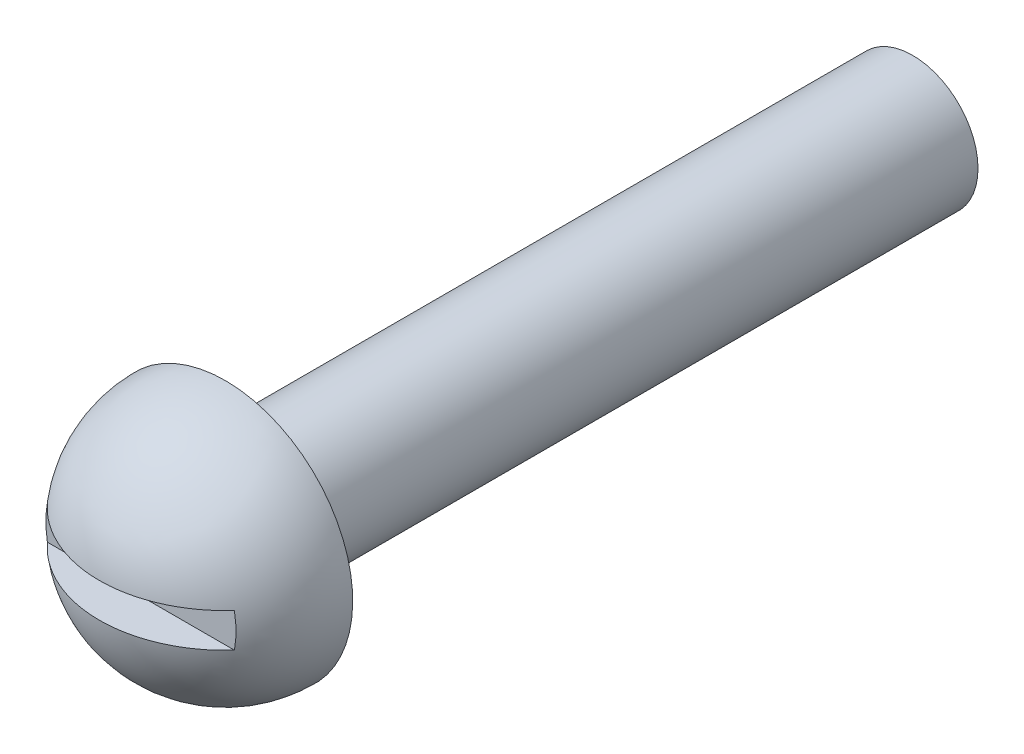
SolidWorks part; units mm, degrees
material "Plain Carbon Steel"
ref_plane "Front Plane" through (0, 0, 0) normal (0, 0, 1) x (1, 0, 0)
ref_plane "Top Plane" through (0, 0, 0) normal (0, 1, 0) x (1, 0, 0)
ref_plane "Right Plane" through (0, 0, 0) normal (1, 0, 0) x (0, 0, -1)
sketch "Shank Profile Ø0.19" plane through (0, 0, 0) normal (0, 0, 1) x (1, 0, 0)
  circle A0 centre (0, 0) radius 2.413
  dimension "D1" = 4.826
extrude "Shank" add sketch "Shank Profile Ø0.19" along normal blind 25.4
sketch "Round Head Profile" plane through (0, 0, 0) normal (1, 0, 0) x (0, 0, -1)
  line L0 (-25.4, 0) -> (-33.5003, 0) construction
  line L1 (-25.4, 2.413) -> (-25.4, -2.413) construction
  line L2 (-25.4, 0) -> (-25.4, 4.7028)
  line L3 (-30.1028, 0) -> (-25.4, 0)
  arc A0 (-25.4, 4.7028) -> (-30.1028, 0) centre (-25.4, 0) ccw
  dimension "D1" = 4.7028
  dimension "D2" = 4.7028
revolve "Round Head" add sketch "Round Head Profile" angle 360 about L0
sketch "Screwdriver Slot Profile" plane through (0, 0, 0) normal (1, 0, 0) x (0, 0, -1)
  line L1 (-31.0653, 0.635) -> (-28.5253, 0.635)
  line L2 (-31.0653, 0.635) -> (-31.0653, -0.635)
  line L3 (-31.0653, -0.635) -> (-28.5253, -0.635)
  line L4 (-28.5253, 0.635) -> (-28.5253, -0.635)
  point P4 (-31.0653, 0)
  dimension "D1" = 1.27
  dimension "D2" = 2.54
  dimension "D3" = 31.0653
extrude "Screwdriver Slot" cut sketch "Screwdriver Slot Profile" against normal through all both and the other way through all
